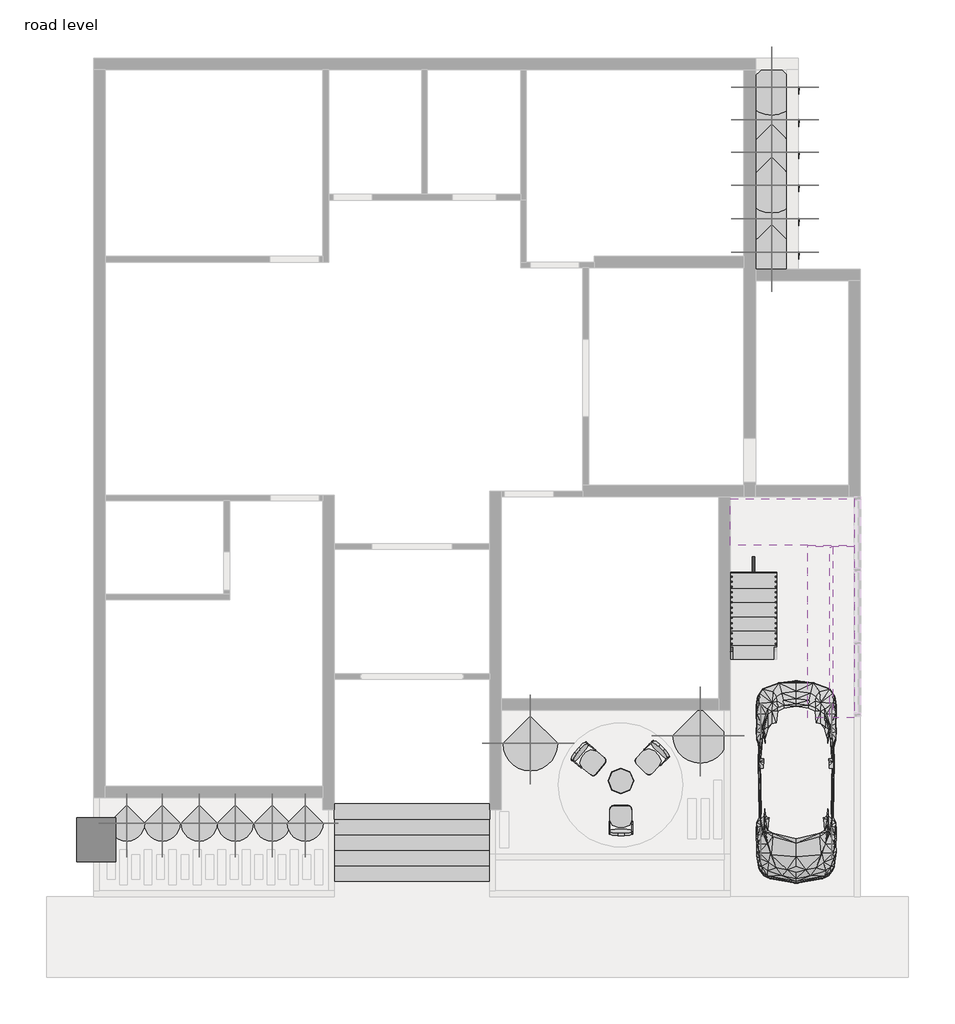
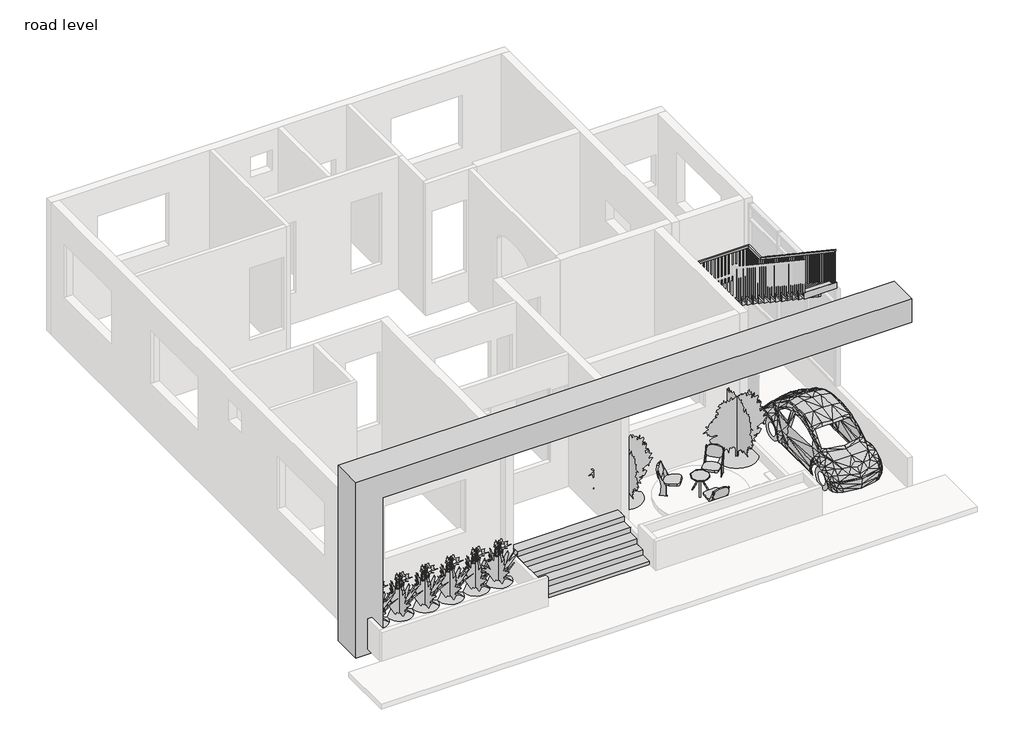
# One storey, part 3 of 3: 14 geographic elements, 6 furniture elements, 2 members, 2 stair flights, 1 proxy, 1 railing, 1 slab.
"""IFC4 building model written with IfcOpenShell, lengths in millimetres."""

from ifc_helpers import new_model, si_unit, frame, origin, place, context, project, spatial, polyline, outline, extrude, faceted_brep, transform, mapped, element, save
from components import rpc_beetle_rpc_beetle_31f8b51e, casework_1_casework_1_0b0e07b3, casework_2_casework_2_4a4ec244, furniture_eb3a3c23, furniture_9d41381f, rpc_plant_tropical_5a024449, rpc_plant_tropical_japanese_fern_2_5_15da35ff, rpc_plant_tropical_jungle_flame_3_a18473df, non_monolithic_landing_47fb7adf, stair_flight_c2955f1a, stair_flight_52fba82a

model = new_model("IFC4")

# Units and contexts
model_context = context("Model", 3, world=origin())
ifc_project = project(units=[si_unit("LENGTHUNIT", "METRE", prefix="MILLI")], contexts=[model_context])

# Site, building, storey
site = spatial("IfcSite", under=ifc_project)
building = spatial("IfcBuilding", under=site)
storey = spatial("IfcBuildingStorey", under=building, Name="road level", Elevation=0.0)

# Proxy
placement = place(None, origin())
rpc_beetle_rpc_beetle_shape = rpc_beetle_rpc_beetle_31f8b51e(model_context)
element("IfcBuildingElementProxy", 1, Name="RPC Beetle : RPC Beetle", ObjectType="RPC Beetle : RPC Beetle", at=placement, inside=storey, context=model_context, shape_type="MappedRepresentation", body=[
    mapped(rpc_beetle_rpc_beetle_shape, transform((-6377.2994093, 2324.2737487, 0.0), x_axis=(-1.0, 0.0, 0.0), y_axis=(0.0, -1.0, 0.0), z_axis=(0.0, 0.0, 1.0))),
])

# Furniture
casework_1_casework_1_shape = casework_1_casework_1_0b0e07b3(model_context)
element("IfcFurniture", 2, ObjectType="Casework 1 : Casework 1", at=placement, inside=storey, context=model_context, shape_type="MappedRepresentation", body=[
    mapped(casework_1_casework_1_shape, transform((0.0, 120.65, -1549.4), x_axis=(1.0, 0.0, 0.0), y_axis=(0.0, 1.0, 0.0), z_axis=(0.0, 0.0, 1.0))),
])
casework_2_casework_2_shape = casework_2_casework_2_4a4ec244(model_context)
element("IfcFurniture", 3, ObjectType="Casework 2 : Casework 2", at=placement, inside=storey, context=model_context, shape_type="MappedRepresentation", body=[
    mapped(casework_2_casework_2_shape, transform((0.0, 0.0, 0.0), x_axis=(1.0, 0.0, 0.0), y_axis=(0.0, 1.0, 0.0), z_axis=(0.0, 0.0, 1.0))),
])
furniture_shape = furniture_eb3a3c23(model_context)
element("IfcFurniture", 4, ObjectType="Seating-Auditorium : 18\" x 24\" x 30\"", at=placement, inside=storey, context=model_context, shape_type="MappedRepresentation", body=[
    mapped(furniture_shape, transform((-10501.2884503, 1788.2599183, 127.0), x_axis=(-0.6326906073859195, -0.7744046715546312, 0.0), y_axis=(0.7744046715546312, -0.6326906073859195, 0.0), z_axis=(0.0, 0.0, 1.0))),
])
element("IfcFurniture", 5, ObjectType="Seating-Auditorium : 18\" x 24\" x 30\"", at=placement, inside=storey, context=model_context, shape_type="MappedRepresentation", body=[
    mapped(furniture_shape, transform((-9979.7272781, 134.5837076, 127.0), x_axis=(1.0, 0.0, 0.0), y_axis=(0.0, 1.0, 0.0), z_axis=(0.0, 0.0, 1.0))),
])
element("IfcFurniture", 6, ObjectType="Seating-Auditorium : 18\" x 24\" x 30\"", at=placement, inside=storey, context=model_context, shape_type="MappedRepresentation", body=[
    mapped(furniture_shape, transform((-8958.0647625, 1589.6695414, 127.0), x_axis=(-0.7071067811865437, 0.7071067811865515, 0.0), y_axis=(-0.7071067811865515, -0.7071067811865437, 0.0), z_axis=(0.0, 0.0, 1.0))),
])
furniture_2_shape = furniture_9d41381f(model_context)
element("IfcFurniture", 7, ObjectType="Table-Trio End : 20\" Diameter", at=placement, inside=storey, context=model_context, shape_type="MappedRepresentation", body=[
    mapped(furniture_2_shape, transform((-9818.9994093, 1111.8591175, 127.0), x_axis=(1.0, 0.0, 0.0), y_axis=(0.0, 1.0, 0.0), z_axis=(0.0, 0.0, 1.0))),
])

# Geographic elements
rpc_plant_tropical_shape = rpc_plant_tropical_5a024449(model_context)
element("IfcGeographicElement", 8, ObjectType="RPC Plant - Tropical", at=placement, inside=storey, context=model_context, shape_type="MappedRepresentation", body=[
    mapped(rpc_plant_tropical_shape, transform((-19521.7994093, 285.9237487, 152.4), x_axis=(1.0, 0.0, 0.0), y_axis=(0.0, 1.0, 0.0), z_axis=(0.0, 0.0, 1.0))),
])
element("IfcGeographicElement", 9, ObjectType="RPC Plant - Tropical", at=placement, inside=storey, context=model_context, shape_type="MappedRepresentation", body=[
    mapped(rpc_plant_tropical_shape, transform((-18823.2994093, 285.9237487, 152.4), x_axis=(1.0, 0.0, 0.0), y_axis=(0.0, 1.0, 0.0), z_axis=(0.0, 0.0, 1.0))),
])
element("IfcGeographicElement", 10, ObjectType="RPC Plant - Tropical", at=placement, inside=storey, context=model_context, shape_type="MappedRepresentation", body=[
    mapped(rpc_plant_tropical_shape, transform((-16016.5994093, 285.9237487, 152.4), x_axis=(1.0, 0.0, 0.0), y_axis=(0.0, 1.0, 0.0), z_axis=(0.0, 0.0, 1.0))),
])
element("IfcGeographicElement", 11, ObjectType="RPC Plant - Tropical", at=placement, inside=storey, context=model_context, shape_type="MappedRepresentation", body=[
    mapped(rpc_plant_tropical_shape, transform((-16664.2994093, 285.9237487, 152.4), x_axis=(1.0, 0.0, 0.0), y_axis=(0.0, 1.0, 0.0), z_axis=(0.0, 0.0, 1.0))),
])
element("IfcGeographicElement", 12, ObjectType="RPC Plant - Tropical", at=placement, inside=storey, context=model_context, shape_type="MappedRepresentation", body=[
    mapped(rpc_plant_tropical_shape, transform((-17387.2102356, 285.9237487, 152.4), x_axis=(1.0, 0.0, 0.0), y_axis=(0.0, 1.0, 0.0), z_axis=(0.0, 0.0, 1.0))),
])
element("IfcGeographicElement", 13, ObjectType="RPC Plant - Tropical", at=placement, inside=storey, context=model_context, shape_type="MappedRepresentation", body=[
    mapped(rpc_plant_tropical_shape, transform((-18100.388583, 285.9237487, 152.4), x_axis=(1.0, 0.0, 0.0), y_axis=(0.0, 1.0, 0.0), z_axis=(0.0, 0.0, 1.0))),
])
rpc_plant_tropical_japanese_fern_2_5_shape = rpc_plant_tropical_japanese_fern_2_5_15da35ff(model_context)
element("IfcGeographicElement", 14, ObjectType="RPC Plant - Tropical : Japanese Fern - 2.5'", at=placement, inside=storey, context=model_context, shape_type="MappedRepresentation", body=[
    mapped(rpc_plant_tropical_japanese_fern_2_5_shape, transform((-6859.8994093, 14725.8237487, 127.0), x_axis=(1.0, 0.0, 0.0), y_axis=(0.0, 1.0, 0.0), z_axis=(0.0, 0.0, 1.0))),
])
element("IfcGeographicElement", 15, ObjectType="RPC Plant - Tropical : Japanese Fern - 2.5'", at=placement, inside=storey, context=model_context, shape_type="MappedRepresentation", body=[
    mapped(rpc_plant_tropical_japanese_fern_2_5_shape, transform((-6859.8994093, 14090.8237487, 127.0), x_axis=(1.0, 0.0, 0.0), y_axis=(0.0, 1.0, 0.0), z_axis=(0.0, 0.0, 1.0))),
])
element("IfcGeographicElement", 16, ObjectType="RPC Plant - Tropical : Japanese Fern - 2.5'", at=placement, inside=storey, context=model_context, shape_type="MappedRepresentation", body=[
    mapped(rpc_plant_tropical_japanese_fern_2_5_shape, transform((-6859.8994093, 13455.8237487, 127.0), x_axis=(1.0, 0.0, 0.0), y_axis=(0.0, 1.0, 0.0), z_axis=(0.0, 0.0, 1.0))),
])
element("IfcGeographicElement", 17, ObjectType="RPC Plant - Tropical : Japanese Fern - 2.5'", at=placement, inside=storey, context=model_context, shape_type="MappedRepresentation", body=[
    mapped(rpc_plant_tropical_japanese_fern_2_5_shape, transform((-6859.8994093, 12808.1237487, 127.0), x_axis=(1.0, 0.0, 0.0), y_axis=(0.0, 1.0, 0.0), z_axis=(0.0, 0.0, 1.0))),
])
element("IfcGeographicElement", 18, ObjectType="RPC Plant - Tropical : Japanese Fern - 2.5'", at=placement, inside=storey, context=model_context, shape_type="MappedRepresentation", body=[
    mapped(rpc_plant_tropical_japanese_fern_2_5_shape, transform((-6859.8994093, 12147.7237487, 127.0), x_axis=(1.0, 0.0, 0.0), y_axis=(0.0, 1.0, 0.0), z_axis=(0.0, 0.0, 1.0))),
])
element("IfcGeographicElement", 19, ObjectType="RPC Plant - Tropical : Japanese Fern - 2.5'", at=placement, inside=storey, context=model_context, shape_type="MappedRepresentation", body=[
    mapped(rpc_plant_tropical_japanese_fern_2_5_shape, transform((-6859.8994093, 11487.3237487, 127.0), x_axis=(1.0, 0.0, 0.0), y_axis=(0.0, 1.0, 0.0), z_axis=(0.0, 0.0, 1.0))),
])
rpc_plant_tropical_jungle_flame_3_shape = rpc_plant_tropical_jungle_flame_3_a18473df(model_context)
element("IfcGeographicElement", 20, ObjectType="RPC Plant - Tropical : Jungle Flame - 3'", at=placement, inside=storey, context=model_context, shape_type="MappedRepresentation", body=[
    mapped(rpc_plant_tropical_jungle_flame_3_shape, transform((-11596.9994093, 1848.0237487, 127.0), x_axis=(1.0, 0.0, 0.0), y_axis=(0.0, 1.0, 0.0), z_axis=(0.0, 0.0, 1.0))),
])
element("IfcGeographicElement", 21, ObjectType="RPC Plant - Tropical : Jungle Flame - 3'", at=placement, inside=storey, context=model_context, shape_type="MappedRepresentation", body=[
    mapped(rpc_plant_tropical_jungle_flame_3_shape, transform((-8261.3350514, 2000.4237487, 127.0), x_axis=(1.0, 0.0, 0.0), y_axis=(0.0, 1.0, 0.0), z_axis=(0.0, 0.0, 1.0))),
])

# Members
element("IfcMember", 22, ObjectType="Carriage - 2\" Width", at=placement, inside=storey, context=model_context, shape_type="SweptSolid", body=[
    extrude(outline(polyline([(5734.2237487, 1445.4909091), (5734.2237487, 1347.8221019), (3720.8104853, 0.0), (3530.7737487, 0.0), (3530.7737487, 136.2363636), (3810.1737487, 136.2363636), (3810.1737487, 323.2727273), (4089.5737487, 323.2727273), (4089.5737487, 510.3090909), (4368.9737487, 510.3090909), (4368.9737487, 697.3454545), (4648.3737487, 697.3454545), (4648.3737487, 884.3818182), (4927.7737487, 884.3818182), (4927.7737487, 1071.4181818), (5207.1737487, 1071.4181818), (5207.1737487, 1258.4545455), (5486.5737487, 1258.4545455), (5486.5737487, 1445.4909091), (5734.2237487, 1445.4909091)])), frame((-7240.8994093, 0.0, 0.0), z_axis=(1.0, 0.0, 0.0), x_axis=(0.0, 1.0, 0.0)), (0.0, 0.0, 1.0), 50.8),
])
element("IfcMember", 23, ObjectType="Carriage - 2\" Width", at=placement, inside=storey, context=model_context, shape_type="SweptSolid", body=[
    extrude(outline(polyline([(2381.4237487, 3779.2948292), (2381.4237487, 3876.9636364), (2629.0737487, 3876.9636364), (2629.0737487, 3689.9272727), (2908.4737487, 3689.9272727), (2908.4737487, 3502.8909091), (3187.8737487, 3502.8909091), (3187.8737487, 3315.8545455), (3467.2737487, 3315.8545455), (3467.2737487, 3128.8181818), (3746.6737487, 3128.8181818), (3746.6737487, 2941.7818182), (4026.0737487, 2941.7818182), (4026.0737487, 2754.7454545), (4305.4737487, 2754.7454545), (4305.4737487, 2567.7090909), (4584.8737487, 2567.7090909), (4584.8737487, 2380.6727273), (4864.2737487, 2380.6727273), (4864.2737487, 2193.6363636), (5143.6737487, 2193.6363636), (5143.6737487, 2006.6), (5423.0737487, 2006.6), (5423.0737487, 1819.5636364), (5702.4737487, 1819.5636364), (5702.4737487, 1556.1125978), (2381.4237487, 3779.2948292)])), frame((-5716.8994093, 0.0, 0.0), z_axis=(1.0, 0.0, 0.0), x_axis=(0.0, 1.0, 0.0)), (0.0, 0.0, 1.0), 50.8),
])

# Railing
element("IfcRailing", 24, ObjectType="Handrail - Rectangular", at=placement, inside=storey, context=model_context, shape_type="SolidModel", body=[
    faceted_brep([(-7672.6994093, 3499.0237487, 1101.4363636), (-7672.6994093, 3499.0237487, 1040.3046237), (-7621.8994093, 3499.0237487, 1040.3046237), (-7621.8994093, 3499.0237487, 1101.4363636), (-7672.6994093, 5734.2237487, 2597.7272727), (-7672.6994093, 5749.6575825, 2546.9272727), (-7621.8994093, 5749.6575825, 2546.9272727), (-7621.8994093, 5734.2237487, 2597.7272727), (-7672.6994093, 6648.6237487, 2597.7272727), (-7672.6994093, 6648.6237487, 2546.9272727), (-7621.8994093, 6597.8237487, 2546.9272727), (-7621.8994093, 6597.8237487, 2597.7272727), (-5234.2994093, 6648.6237487, 2597.7272727), (-5234.2994093, 6648.6237487, 2546.9272727), (-5285.0994093, 6597.8237487, 2546.9272727), (-5285.0994093, 6597.8237487, 2597.7272727), (-5234.2994093, 6013.6237487, 2597.7272727), (-5234.2994093, 5998.1899149, 2546.9272727), (-5285.0994093, 5998.1899149, 2546.9272727), (-5285.0994093, 6013.6237487, 2597.7272727), (-5234.2994093, 5734.2237487, 2784.7636364), (-5234.2994093, 5705.9645192, 2742.5492318), (-5285.0994093, 5705.9645192, 2742.5492318), (-5285.0994093, 5734.2237487, 2784.7636364), (-5234.2994093, 2381.4237487, 5029.2), (-5285.0994093, 2381.4237487, 5029.2), (-5285.0994093, 2381.4237487, 4968.06826), (-5234.2994093, 2381.4237487, 4968.06826)], [[[0, 1, 2, 3]], [[1, 0, 4, 5]], [[2, 1, 5, 6]], [[3, 2, 6, 7]], [[0, 3, 7, 4]], [[5, 4, 8, 9]], [[6, 5, 9, 10]], [[7, 6, 10, 11]], [[4, 7, 11, 8]], [[9, 8, 12, 13]], [[10, 9, 13, 14]], [[11, 10, 14, 15]], [[8, 11, 15, 12]], [[13, 12, 16, 17]], [[14, 13, 17, 18]], [[15, 14, 18, 19]], [[12, 15, 19, 16]], [[17, 16, 20, 21]], [[18, 17, 21, 22]], [[19, 18, 22, 23]], [[16, 19, 23, 20]], [[24, 25, 26, 27]], [[21, 20, 24, 27]], [[22, 21, 27, 26]], [[23, 22, 26, 25]], [[20, 23, 25, 24]]]),
    extrude(outline(polyline([(2492.5487487, 4893.6787972), (2492.5487487, 3927.7636364), (2473.4987487, 3927.7636364), (2473.4987487, 4906.4312766), (2492.5487487, 4893.6787972)])), frame((-5269.2244093, 0.0, 0.0), z_axis=(1.0, 0.0, 0.0), x_axis=(0.0, 1.0, 0.0)), (0.0, 0.0, 1.0), 19.05),
    extrude(outline(polyline([(2594.1487487, 4825.6655741), (2594.1487487, 3927.7636364), (2575.0987487, 3927.7636364), (2575.0987487, 4838.4180534), (2594.1487487, 4825.6655741)])), frame((-5269.2244093, 0.0, 0.0), z_axis=(1.0, 0.0, 0.0), x_axis=(0.0, 1.0, 0.0)), (0.0, 0.0, 1.0), 19.05),
    extrude(outline(polyline([(2695.7487487, 4757.6523509), (2695.7487487, 3740.7272727), (2676.6987487, 3740.7272727), (2676.6987487, 4770.4048303), (2695.7487487, 4757.6523509)])), frame((-5269.2244093, 0.0, 0.0), z_axis=(1.0, 0.0, 0.0), x_axis=(0.0, 1.0, 0.0)), (0.0, 0.0, 1.0), 19.05),
    extrude(outline(polyline([(2797.3487487, 4689.6391278), (2797.3487487, 3740.7272727), (2778.2987487, 3740.7272727), (2778.2987487, 4702.3916071), (2797.3487487, 4689.6391278)])), frame((-5269.2244093, 0.0, 0.0), z_axis=(1.0, 0.0, 0.0), x_axis=(0.0, 1.0, 0.0)), (0.0, 0.0, 1.0), 19.05),
    extrude(outline(polyline([(2898.9487487, 4621.6259047), (2898.9487487, 3740.7272727), (2879.8987487, 3740.7272727), (2879.8987487, 4634.378384), (2898.9487487, 4621.6259047)])), frame((-5269.2244093, 0.0, 0.0), z_axis=(1.0, 0.0, 0.0), x_axis=(0.0, 1.0, 0.0)), (0.0, 0.0, 1.0), 19.05),
    extrude(outline(polyline([(3000.5487487, 4553.6126815), (3000.5487487, 3553.6909091), (2981.4987487, 3553.6909091), (2981.4987487, 4566.3651609), (3000.5487487, 4553.6126815)])), frame((-5269.2244093, 0.0, 0.0), z_axis=(1.0, 0.0, 0.0), x_axis=(0.0, 1.0, 0.0)), (0.0, 0.0, 1.0), 19.05),
    extrude(outline(polyline([(3102.1487487, 4485.5994584), (3102.1487487, 3553.6909091), (3083.0987487, 3553.6909091), (3083.0987487, 4498.3519377), (3102.1487487, 4485.5994584)])), frame((-5269.2244093, 0.0, 0.0), z_axis=(1.0, 0.0, 0.0), x_axis=(0.0, 1.0, 0.0)), (0.0, 0.0, 1.0), 19.05),
    extrude(outline(polyline([(3203.7487487, 4417.5862352), (3203.7487487, 3553.6909091), (3184.6987487, 3553.6909091), (3184.6987487, 4430.3387146), (3203.7487487, 4417.5862352)])), frame((-5269.2244093, 0.0, 0.0), z_axis=(1.0, 0.0, 0.0), x_axis=(0.0, 1.0, 0.0)), (0.0, 0.0, 1.0), 19.05),
    extrude(outline(polyline([(3305.3487487, 4349.5730121), (3305.3487487, 3366.6545455), (3286.2987487, 3366.6545455), (3286.2987487, 4362.3254914), (3305.3487487, 4349.5730121)])), frame((-5269.2244093, 0.0, 0.0), z_axis=(1.0, 0.0, 0.0), x_axis=(0.0, 1.0, 0.0)), (0.0, 0.0, 1.0), 19.05),
    extrude(outline(polyline([(3406.9487487, 4281.559789), (3406.9487487, 3366.6545455), (3387.8987487, 3366.6545455), (3387.8987487, 4294.3122683), (3406.9487487, 4281.559789)])), frame((-5269.2244093, 0.0, 0.0), z_axis=(1.0, 0.0, 0.0), x_axis=(0.0, 1.0, 0.0)), (0.0, 0.0, 1.0), 19.05),
    extrude(outline(polyline([(3508.5487487, 4213.5465658), (3508.5487487, 3366.6545455), (3489.4987487, 3366.6545455), (3489.4987487, 4226.2990452), (3508.5487487, 4213.5465658)])), frame((-5269.2244093, 0.0, 0.0), z_axis=(1.0, 0.0, 0.0), x_axis=(0.0, 1.0, 0.0)), (0.0, 0.0, 1.0), 19.05),
    extrude(outline(polyline([(3610.1487487, 4145.5333427), (3610.1487487, 3179.6181818), (3591.0987487, 3179.6181818), (3591.0987487, 4158.285822), (3610.1487487, 4145.5333427)])), frame((-5269.2244093, 0.0, 0.0), z_axis=(1.0, 0.0, 0.0), x_axis=(0.0, 1.0, 0.0)), (0.0, 0.0, 1.0), 19.05),
    extrude(outline(polyline([(3711.7487487, 4077.5201195), (3711.7487487, 3179.6181818), (3692.6987487, 3179.6181818), (3692.6987487, 4090.2725989), (3711.7487487, 4077.5201195)])), frame((-5269.2244093, 0.0, 0.0), z_axis=(1.0, 0.0, 0.0), x_axis=(0.0, 1.0, 0.0)), (0.0, 0.0, 1.0), 19.05),
    extrude(outline(polyline([(3813.3487487, 4009.5068964), (3813.3487487, 2992.5818182), (3794.2987487, 2992.5818182), (3794.2987487, 4022.2593757), (3813.3487487, 4009.5068964)])), frame((-5269.2244093, 0.0, 0.0), z_axis=(1.0, 0.0, 0.0), x_axis=(0.0, 1.0, 0.0)), (0.0, 0.0, 1.0), 19.05),
    extrude(outline(polyline([(3914.9487487, 3941.4936733), (3914.9487487, 2992.5818182), (3895.8987487, 2992.5818182), (3895.8987487, 3954.2461526), (3914.9487487, 3941.4936733)])), frame((-5269.2244093, 0.0, 0.0), z_axis=(1.0, 0.0, 0.0), x_axis=(0.0, 1.0, 0.0)), (0.0, 0.0, 1.0), 19.05),
    extrude(outline(polyline([(4016.5487487, 3873.4804501), (4016.5487487, 2992.5818182), (3997.4987487, 2992.5818182), (3997.4987487, 3886.2329295), (4016.5487487, 3873.4804501)])), frame((-5269.2244093, 0.0, 0.0), z_axis=(1.0, 0.0, 0.0), x_axis=(0.0, 1.0, 0.0)), (0.0, 0.0, 1.0), 19.05),
    extrude(outline(polyline([(4118.1487487, 3805.467227), (4118.1487487, 2805.5454545), (4099.0987487, 2805.5454545), (4099.0987487, 3818.2197063), (4118.1487487, 3805.467227)])), frame((-5269.2244093, 0.0, 0.0), z_axis=(1.0, 0.0, 0.0), x_axis=(0.0, 1.0, 0.0)), (0.0, 0.0, 1.0), 19.05),
    extrude(outline(polyline([(4219.7487487, 3737.4540038), (4219.7487487, 2805.5454545), (4200.6987487, 2805.5454545), (4200.6987487, 3750.2064832), (4219.7487487, 3737.4540038)])), frame((-5269.2244093, 0.0, 0.0), z_axis=(1.0, 0.0, 0.0), x_axis=(0.0, 1.0, 0.0)), (0.0, 0.0, 1.0), 19.05),
    extrude(outline(polyline([(4321.3487487, 3669.4407807), (4321.3487487, 2805.5454545), (4302.2987487, 2805.5454545), (4302.2987487, 3682.19326), (4321.3487487, 3669.4407807)])), frame((-5269.2244093, 0.0, 0.0), z_axis=(1.0, 0.0, 0.0), x_axis=(0.0, 1.0, 0.0)), (0.0, 0.0, 1.0), 19.05),
    extrude(outline(polyline([(4422.9487487, 3601.4275576), (4422.9487487, 2618.5090909), (4403.8987487, 2618.5090909), (4403.8987487, 3614.1800369), (4422.9487487, 3601.4275576)])), frame((-5269.2244093, 0.0, 0.0), z_axis=(1.0, 0.0, 0.0), x_axis=(0.0, 1.0, 0.0)), (0.0, 0.0, 1.0), 19.05),
    extrude(outline(polyline([(4524.5487487, 3533.4143344), (4524.5487487, 2618.5090909), (4505.4987487, 2618.5090909), (4505.4987487, 3546.1668138), (4524.5487487, 3533.4143344)])), frame((-5269.2244093, 0.0, 0.0), z_axis=(1.0, 0.0, 0.0), x_axis=(0.0, 1.0, 0.0)), (0.0, 0.0, 1.0), 19.05),
    extrude(outline(polyline([(4626.1487487, 3465.4011113), (4626.1487487, 2618.5090909), (4607.0987487, 2618.5090909), (4607.0987487, 3478.1535906), (4626.1487487, 3465.4011113)])), frame((-5269.2244093, 0.0, 0.0), z_axis=(1.0, 0.0, 0.0), x_axis=(0.0, 1.0, 0.0)), (0.0, 0.0, 1.0), 19.05),
    extrude(outline(polyline([(4727.7487487, 3397.3878881), (4727.7487487, 2431.4727273), (4708.6987487, 2431.4727273), (4708.6987487, 3410.1403675), (4727.7487487, 3397.3878881)])), frame((-5269.2244093, 0.0, 0.0), z_axis=(1.0, 0.0, 0.0), x_axis=(0.0, 1.0, 0.0)), (0.0, 0.0, 1.0), 19.05),
    extrude(outline(polyline([(4829.3487487, 3329.374665), (4829.3487487, 2431.4727273), (4810.2987487, 2431.4727273), (4810.2987487, 3342.1271443), (4829.3487487, 3329.374665)])), frame((-5269.2244093, 0.0, 0.0), z_axis=(1.0, 0.0, 0.0), x_axis=(0.0, 1.0, 0.0)), (0.0, 0.0, 1.0), 19.05),
    extrude(outline(polyline([(4930.9487487, 3261.3614419), (4930.9487487, 2244.4363636), (4911.8987487, 2244.4363636), (4911.8987487, 3274.1139212), (4930.9487487, 3261.3614419)])), frame((-5269.2244093, 0.0, 0.0), z_axis=(1.0, 0.0, 0.0), x_axis=(0.0, 1.0, 0.0)), (0.0, 0.0, 1.0), 19.05),
    extrude(outline(polyline([(5032.5487487, 3193.3482187), (5032.5487487, 2244.4363636), (5013.4987487, 2244.4363636), (5013.4987487, 3206.1006981), (5032.5487487, 3193.3482187)])), frame((-5269.2244093, 0.0, 0.0), z_axis=(1.0, 0.0, 0.0), x_axis=(0.0, 1.0, 0.0)), (0.0, 0.0, 1.0), 19.05),
    extrude(outline(polyline([(5134.1487487, 3125.3349956), (5134.1487487, 2244.4363636), (5115.0987487, 2244.4363636), (5115.0987487, 3138.0874749), (5134.1487487, 3125.3349956)])), frame((-5269.2244093, 0.0, 0.0), z_axis=(1.0, 0.0, 0.0), x_axis=(0.0, 1.0, 0.0)), (0.0, 0.0, 1.0), 19.05),
    extrude(outline(polyline([(5235.7487487, 3057.3217724), (5235.7487487, 2057.4), (5216.6987487, 2057.4), (5216.6987487, 3070.0742518), (5235.7487487, 3057.3217724)])), frame((-5269.2244093, 0.0, 0.0), z_axis=(1.0, 0.0, 0.0), x_axis=(0.0, 1.0, 0.0)), (0.0, 0.0, 1.0), 19.05),
    extrude(outline(polyline([(5337.3487487, 2989.3085493), (5337.3487487, 2057.4), (5318.2987487, 2057.4), (5318.2987487, 3002.0610286), (5337.3487487, 2989.3085493)])), frame((-5269.2244093, 0.0, 0.0), z_axis=(1.0, 0.0, 0.0), x_axis=(0.0, 1.0, 0.0)), (0.0, 0.0, 1.0), 19.05),
    extrude(outline(polyline([(5438.9487487, 2921.2953262), (5438.9487487, 2057.4), (5419.8987487, 2057.4), (5419.8987487, 2934.0478055), (5438.9487487, 2921.2953262)])), frame((-5269.2244093, 0.0, 0.0), z_axis=(1.0, 0.0, 0.0), x_axis=(0.0, 1.0, 0.0)), (0.0, 0.0, 1.0), 19.05),
    extrude(outline(polyline([(5540.5487487, 2853.282103), (5540.5487487, 1870.3636364), (5521.4987487, 1870.3636364), (5521.4987487, 2866.0345824), (5540.5487487, 2853.282103)])), frame((-5269.2244093, 0.0, 0.0), z_axis=(1.0, 0.0, 0.0), x_axis=(0.0, 1.0, 0.0)), (0.0, 0.0, 1.0), 19.05),
    extrude(outline(polyline([(5642.1487487, 2785.2688799), (5642.1487487, 1870.3636364), (5623.0987487, 1870.3636364), (5623.0987487, 2798.0213592), (5642.1487487, 2785.2688799)])), frame((-5269.2244093, 0.0, 0.0), z_axis=(1.0, 0.0, 0.0), x_axis=(0.0, 1.0, 0.0)), (0.0, 0.0, 1.0), 19.05),
    extrude(outline(polyline([(5819.9487487, 2666.2457394), (5819.9487487, 1683.3272727), (5800.8987487, 1683.3272727), (5800.8987487, 2678.9982187), (5819.9487487, 2666.2457394)])), frame((-5269.2244093, 0.0, 0.0), z_axis=(1.0, 0.0, 0.0), x_axis=(0.0, 1.0, 0.0)), (0.0, 0.0, 1.0), 19.05),
    extrude(outline(polyline([(5921.5487487, 2598.2325162), (5921.5487487, 1683.3272727), (5902.4987487, 1683.3272727), (5902.4987487, 2610.9849956), (5921.5487487, 2598.2325162)])), frame((-5269.2244093, 0.0, 0.0), z_axis=(1.0, 0.0, 0.0), x_axis=(0.0, 1.0, 0.0)), (0.0, 0.0, 1.0), 19.05),
    extrude(outline(polyline([(-5250.1744093, 6023.1487487), (-5250.1744093, 6004.0987487), (-5269.2244093, 6004.0987487), (-5269.2244093, 6023.1487487), (-5250.1744093, 6023.1487487)])), frame((0.0, 0.0, 1683.3272727), z_axis=(0.0, 0.0, 1.0), x_axis=(1.0, 0.0, 0.0)), (0.0, 0.0, 1.0), 863.6),
    extrude(outline(polyline([(-5250.1744093, 6124.7487487), (-5250.1744093, 6105.6987487), (-5269.2244093, 6105.6987487), (-5269.2244093, 6124.7487487), (-5250.1744093, 6124.7487487)])), frame((0.0, 0.0, 1683.3272727), z_axis=(0.0, 0.0, 1.0), x_axis=(1.0, 0.0, 0.0)), (0.0, 0.0, 1.0), 863.6),
    extrude(outline(polyline([(-5250.1744093, 6226.3487487), (-5250.1744093, 6207.2987487), (-5269.2244093, 6207.2987487), (-5269.2244093, 6226.3487487), (-5250.1744093, 6226.3487487)])), frame((0.0, 0.0, 1683.3272727), z_axis=(0.0, 0.0, 1.0), x_axis=(1.0, 0.0, 0.0)), (0.0, 0.0, 1.0), 863.6),
    extrude(outline(polyline([(-5250.1744093, 6327.9487487), (-5250.1744093, 6308.8987487), (-5269.2244093, 6308.8987487), (-5269.2244093, 6327.9487487), (-5250.1744093, 6327.9487487)])), frame((0.0, 0.0, 1683.3272727), z_axis=(0.0, 0.0, 1.0), x_axis=(1.0, 0.0, 0.0)), (0.0, 0.0, 1.0), 863.6),
    extrude(outline(polyline([(-5250.1744093, 6429.5487487), (-5250.1744093, 6410.4987487), (-5269.2244093, 6410.4987487), (-5269.2244093, 6429.5487487), (-5250.1744093, 6429.5487487)])), frame((0.0, 0.0, 1683.3272727), z_axis=(0.0, 0.0, 1.0), x_axis=(1.0, 0.0, 0.0)), (0.0, 0.0, 1.0), 863.6),
    extrude(outline(polyline([(-5250.1744093, 6531.1487487), (-5250.1744093, 6512.0987487), (-5269.2244093, 6512.0987487), (-5269.2244093, 6531.1487487), (-5250.1744093, 6531.1487487)])), frame((0.0, 0.0, 1683.3272727), z_axis=(0.0, 0.0, 1.0), x_axis=(1.0, 0.0, 0.0)), (0.0, 0.0, 1.0), 863.6),
    extrude(outline(polyline([(-5320.0244093, 6632.7487487), (-5300.9744093, 6632.7487487), (-5300.9744093, 6613.6987487), (-5320.0244093, 6613.6987487), (-5320.0244093, 6632.7487487)])), frame((0.0, 0.0, 1683.3272727), z_axis=(0.0, 0.0, 1.0), x_axis=(1.0, 0.0, 0.0)), (0.0, 0.0, 1.0), 863.6),
    extrude(outline(polyline([(-5421.6244093, 6632.7487487), (-5402.5744093, 6632.7487487), (-5402.5744093, 6613.6987487), (-5421.6244093, 6613.6987487), (-5421.6244093, 6632.7487487)])), frame((0.0, 0.0, 1683.3272727), z_axis=(0.0, 0.0, 1.0), x_axis=(1.0, 0.0, 0.0)), (0.0, 0.0, 1.0), 863.6),
    extrude(outline(polyline([(-5523.2244093, 6632.7487487), (-5504.1744093, 6632.7487487), (-5504.1744093, 6613.6987487), (-5523.2244093, 6613.6987487), (-5523.2244093, 6632.7487487)])), frame((0.0, 0.0, 1683.3272727), z_axis=(0.0, 0.0, 1.0), x_axis=(1.0, 0.0, 0.0)), (0.0, 0.0, 1.0), 863.6),
    extrude(outline(polyline([(-5624.8244093, 6632.7487487), (-5605.7744093, 6632.7487487), (-5605.7744093, 6613.6987487), (-5624.8244093, 6613.6987487), (-5624.8244093, 6632.7487487)])), frame((0.0, 0.0, 1683.3272727), z_axis=(0.0, 0.0, 1.0), x_axis=(1.0, 0.0, 0.0)), (0.0, 0.0, 1.0), 863.6),
    extrude(outline(polyline([(-5726.4244093, 6632.7487487), (-5707.3744093, 6632.7487487), (-5707.3744093, 6613.6987487), (-5726.4244093, 6613.6987487), (-5726.4244093, 6632.7487487)])), frame((0.0, 0.0, 1683.3272727), z_axis=(0.0, 0.0, 1.0), x_axis=(1.0, 0.0, 0.0)), (0.0, 0.0, 1.0), 863.6),
    extrude(outline(polyline([(-5828.0244093, 6632.7487487), (-5808.9744093, 6632.7487487), (-5808.9744093, 6613.6987487), (-5828.0244093, 6613.6987487), (-5828.0244093, 6632.7487487)])), frame((0.0, 0.0, 1683.3272727), z_axis=(0.0, 0.0, 1.0), x_axis=(1.0, 0.0, 0.0)), (0.0, 0.0, 1.0), 863.6),
    extrude(outline(polyline([(-5929.6244093, 6632.7487487), (-5910.5744093, 6632.7487487), (-5910.5744093, 6613.6987487), (-5929.6244093, 6613.6987487), (-5929.6244093, 6632.7487487)])), frame((0.0, 0.0, 1683.3272727), z_axis=(0.0, 0.0, 1.0), x_axis=(1.0, 0.0, 0.0)), (0.0, 0.0, 1.0), 863.6),
    extrude(outline(polyline([(-6031.2244093, 6632.7487487), (-6012.1744093, 6632.7487487), (-6012.1744093, 6613.6987487), (-6031.2244093, 6613.6987487), (-6031.2244093, 6632.7487487)])), frame((0.0, 0.0, 1683.3272727), z_axis=(0.0, 0.0, 1.0), x_axis=(1.0, 0.0, 0.0)), (0.0, 0.0, 1.0), 863.6),
    extrude(outline(polyline([(-6132.8244093, 6632.7487487), (-6113.7744093, 6632.7487487), (-6113.7744093, 6613.6987487), (-6132.8244093, 6613.6987487), (-6132.8244093, 6632.7487487)])), frame((0.0, 0.0, 1683.3272727), z_axis=(0.0, 0.0, 1.0), x_axis=(1.0, 0.0, 0.0)), (0.0, 0.0, 1.0), 863.6),
    extrude(outline(polyline([(-6234.4244093, 6632.7487487), (-6215.3744093, 6632.7487487), (-6215.3744093, 6613.6987487), (-6234.4244093, 6613.6987487), (-6234.4244093, 6632.7487487)])), frame((0.0, 0.0, 1683.3272727), z_axis=(0.0, 0.0, 1.0), x_axis=(1.0, 0.0, 0.0)), (0.0, 0.0, 1.0), 863.6),
    extrude(outline(polyline([(-6336.0244093, 6632.7487487), (-6316.9744093, 6632.7487487), (-6316.9744093, 6613.6987487), (-6336.0244093, 6613.6987487), (-6336.0244093, 6632.7487487)])), frame((0.0, 0.0, 1683.3272727), z_axis=(0.0, 0.0, 1.0), x_axis=(1.0, 0.0, 0.0)), (0.0, 0.0, 1.0), 863.6),
    extrude(outline(polyline([(-6437.6244093, 6632.7487487), (-6418.5744093, 6632.7487487), (-6418.5744093, 6613.6987487), (-6437.6244093, 6613.6987487), (-6437.6244093, 6632.7487487)])), frame((0.0, 0.0, 1683.3272727), z_axis=(0.0, 0.0, 1.0), x_axis=(1.0, 0.0, 0.0)), (0.0, 0.0, 1.0), 863.6),
    extrude(outline(polyline([(-6539.2244093, 6632.7487487), (-6520.1744093, 6632.7487487), (-6520.1744093, 6613.6987487), (-6539.2244093, 6613.6987487), (-6539.2244093, 6632.7487487)])), frame((0.0, 0.0, 1683.3272727), z_axis=(0.0, 0.0, 1.0), x_axis=(1.0, 0.0, 0.0)), (0.0, 0.0, 1.0), 863.6),
    extrude(outline(polyline([(-6640.8244093, 6632.7487487), (-6621.7744093, 6632.7487487), (-6621.7744093, 6613.6987487), (-6640.8244093, 6613.6987487), (-6640.8244093, 6632.7487487)])), frame((0.0, 0.0, 1683.3272727), z_axis=(0.0, 0.0, 1.0), x_axis=(1.0, 0.0, 0.0)), (0.0, 0.0, 1.0), 863.6),
    extrude(outline(polyline([(-6742.4244093, 6632.7487487), (-6723.3744093, 6632.7487487), (-6723.3744093, 6613.6987487), (-6742.4244093, 6613.6987487), (-6742.4244093, 6632.7487487)])), frame((0.0, 0.0, 1683.3272727), z_axis=(0.0, 0.0, 1.0), x_axis=(1.0, 0.0, 0.0)), (0.0, 0.0, 1.0), 863.6),
    extrude(outline(polyline([(-6844.0244093, 6632.7487487), (-6824.9744093, 6632.7487487), (-6824.9744093, 6613.6987487), (-6844.0244093, 6613.6987487), (-6844.0244093, 6632.7487487)])), frame((0.0, 0.0, 1683.3272727), z_axis=(0.0, 0.0, 1.0), x_axis=(1.0, 0.0, 0.0)), (0.0, 0.0, 1.0), 863.6),
    extrude(outline(polyline([(-6945.6244093, 6632.7487487), (-6926.5744093, 6632.7487487), (-6926.5744093, 6613.6987487), (-6945.6244093, 6613.6987487), (-6945.6244093, 6632.7487487)])), frame((0.0, 0.0, 1683.3272727), z_axis=(0.0, 0.0, 1.0), x_axis=(1.0, 0.0, 0.0)), (0.0, 0.0, 1.0), 863.6),
    extrude(outline(polyline([(-7047.2244093, 6632.7487487), (-7028.1744093, 6632.7487487), (-7028.1744093, 6613.6987487), (-7047.2244093, 6613.6987487), (-7047.2244093, 6632.7487487)])), frame((0.0, 0.0, 1683.3272727), z_axis=(0.0, 0.0, 1.0), x_axis=(1.0, 0.0, 0.0)), (0.0, 0.0, 1.0), 863.6),
    extrude(outline(polyline([(-7148.8244093, 6632.7487487), (-7129.7744093, 6632.7487487), (-7129.7744093, 6613.6987487), (-7148.8244093, 6613.6987487), (-7148.8244093, 6632.7487487)])), frame((0.0, 0.0, 1683.3272727), z_axis=(0.0, 0.0, 1.0), x_axis=(1.0, 0.0, 0.0)), (0.0, 0.0, 1.0), 863.6),
    extrude(outline(polyline([(-7250.4244093, 6632.7487487), (-7231.3744093, 6632.7487487), (-7231.3744093, 6613.6987487), (-7250.4244093, 6613.6987487), (-7250.4244093, 6632.7487487)])), frame((0.0, 0.0, 1683.3272727), z_axis=(0.0, 0.0, 1.0), x_axis=(1.0, 0.0, 0.0)), (0.0, 0.0, 1.0), 863.6),
    extrude(outline(polyline([(-7352.0244093, 6632.7487487), (-7332.9744093, 6632.7487487), (-7332.9744093, 6613.6987487), (-7352.0244093, 6613.6987487), (-7352.0244093, 6632.7487487)])), frame((0.0, 0.0, 1683.3272727), z_axis=(0.0, 0.0, 1.0), x_axis=(1.0, 0.0, 0.0)), (0.0, 0.0, 1.0), 863.6),
    extrude(outline(polyline([(-7453.6244093, 6632.7487487), (-7434.5744093, 6632.7487487), (-7434.5744093, 6613.6987487), (-7453.6244093, 6613.6987487), (-7453.6244093, 6632.7487487)])), frame((0.0, 0.0, 1683.3272727), z_axis=(0.0, 0.0, 1.0), x_axis=(1.0, 0.0, 0.0)), (0.0, 0.0, 1.0), 863.6),
    extrude(outline(polyline([(-7555.2244093, 6632.7487487), (-7536.1744093, 6632.7487487), (-7536.1744093, 6613.6987487), (-7555.2244093, 6613.6987487), (-7555.2244093, 6632.7487487)])), frame((0.0, 0.0, 1683.3272727), z_axis=(0.0, 0.0, 1.0), x_axis=(1.0, 0.0, 0.0)), (0.0, 0.0, 1.0), 863.6),
    extrude(outline(polyline([(-7656.8244093, 6537.4987487), (-7656.8244093, 6556.5487487), (-7637.7744093, 6556.5487487), (-7637.7744093, 6537.4987487), (-7656.8244093, 6537.4987487)])), frame((0.0, 0.0, 1683.3272727), z_axis=(0.0, 0.0, 1.0), x_axis=(1.0, 0.0, 0.0)), (0.0, 0.0, 1.0), 863.6),
    extrude(outline(polyline([(-7656.8244093, 6435.8987487), (-7656.8244093, 6454.9487487), (-7637.7744093, 6454.9487487), (-7637.7744093, 6435.8987487), (-7656.8244093, 6435.8987487)])), frame((0.0, 0.0, 1683.3272727), z_axis=(0.0, 0.0, 1.0), x_axis=(1.0, 0.0, 0.0)), (0.0, 0.0, 1.0), 863.6),
    extrude(outline(polyline([(-7656.8244093, 6334.2987487), (-7656.8244093, 6353.3487487), (-7637.7744093, 6353.3487487), (-7637.7744093, 6334.2987487), (-7656.8244093, 6334.2987487)])), frame((0.0, 0.0, 1683.3272727), z_axis=(0.0, 0.0, 1.0), x_axis=(1.0, 0.0, 0.0)), (0.0, 0.0, 1.0), 863.6),
    extrude(outline(polyline([(-7656.8244093, 6232.6987487), (-7656.8244093, 6251.7487487), (-7637.7744093, 6251.7487487), (-7637.7744093, 6232.6987487), (-7656.8244093, 6232.6987487)])), frame((0.0, 0.0, 1683.3272727), z_axis=(0.0, 0.0, 1.0), x_axis=(1.0, 0.0, 0.0)), (0.0, 0.0, 1.0), 863.6),
    extrude(outline(polyline([(-7656.8244093, 6131.0987487), (-7656.8244093, 6150.1487487), (-7637.7744093, 6150.1487487), (-7637.7744093, 6131.0987487), (-7656.8244093, 6131.0987487)])), frame((0.0, 0.0, 1683.3272727), z_axis=(0.0, 0.0, 1.0), x_axis=(1.0, 0.0, 0.0)), (0.0, 0.0, 1.0), 863.6),
    extrude(outline(polyline([(-7656.8244093, 6029.4987487), (-7656.8244093, 6048.5487487), (-7637.7744093, 6048.5487487), (-7637.7744093, 6029.4987487), (-7656.8244093, 6029.4987487)])), frame((0.0, 0.0, 1683.3272727), z_axis=(0.0, 0.0, 1.0), x_axis=(1.0, 0.0, 0.0)), (0.0, 0.0, 1.0), 863.6),
    extrude(outline(polyline([(-7656.8244093, 5927.8987487), (-7656.8244093, 5946.9487487), (-7637.7744093, 5946.9487487), (-7637.7744093, 5927.8987487), (-7656.8244093, 5927.8987487)])), frame((0.0, 0.0, 1683.3272727), z_axis=(0.0, 0.0, 1.0), x_axis=(1.0, 0.0, 0.0)), (0.0, 0.0, 1.0), 863.6),
    extrude(outline(polyline([(-7656.8244093, 5826.2987487), (-7656.8244093, 5845.3487487), (-7637.7744093, 5845.3487487), (-7637.7744093, 5826.2987487), (-7656.8244093, 5826.2987487)])), frame((0.0, 0.0, 1683.3272727), z_axis=(0.0, 0.0, 1.0), x_axis=(1.0, 0.0, 0.0)), (0.0, 0.0, 1.0), 863.6),
    extrude(outline(polyline([(5642.1487487, 2474.9585493), (5642.1487487, 1496.2909091), (5623.0987487, 1496.2909091), (5623.0987487, 2462.20607), (5642.1487487, 2474.9585493)])), frame((-7656.8244093, 0.0, 0.0), z_axis=(1.0, 0.0, 0.0), x_axis=(0.0, 1.0, 0.0)), (0.0, 0.0, 1.0), 19.05),
    extrude(outline(polyline([(5540.5487487, 2406.9453262), (5540.5487487, 1496.2909091), (5521.4987487, 1496.2909091), (5521.4987487, 2394.1928468), (5540.5487487, 2406.9453262)])), frame((-7656.8244093, 0.0, 0.0), z_axis=(1.0, 0.0, 0.0), x_axis=(0.0, 1.0, 0.0)), (0.0, 0.0, 1.0), 19.05),
    extrude(outline(polyline([(5438.9487487, 2338.932103), (5438.9487487, 1309.2545455), (5419.8987487, 1309.2545455), (5419.8987487, 2326.1796237), (5438.9487487, 2338.932103)])), frame((-7656.8244093, 0.0, 0.0), z_axis=(1.0, 0.0, 0.0), x_axis=(0.0, 1.0, 0.0)), (0.0, 0.0, 1.0), 19.05),
    extrude(outline(polyline([(5337.3487487, 2270.9188799), (5337.3487487, 1309.2545455), (5318.2987487, 1309.2545455), (5318.2987487, 2258.1664005), (5337.3487487, 2270.9188799)])), frame((-7656.8244093, 0.0, 0.0), z_axis=(1.0, 0.0, 0.0), x_axis=(0.0, 1.0, 0.0)), (0.0, 0.0, 1.0), 19.05),
    extrude(outline(polyline([(5235.7487487, 2202.9056567), (5235.7487487, 1309.2545455), (5216.6987487, 1309.2545455), (5216.6987487, 2190.1531774), (5235.7487487, 2202.9056567)])), frame((-7656.8244093, 0.0, 0.0), z_axis=(1.0, 0.0, 0.0), x_axis=(0.0, 1.0, 0.0)), (0.0, 0.0, 1.0), 19.05),
    extrude(outline(polyline([(5134.1487487, 2134.8924336), (5134.1487487, 1122.2181818), (5115.0987487, 1122.2181818), (5115.0987487, 2122.1399543), (5134.1487487, 2134.8924336)])), frame((-7656.8244093, 0.0, 0.0), z_axis=(1.0, 0.0, 0.0), x_axis=(0.0, 1.0, 0.0)), (0.0, 0.0, 1.0), 19.05),
    extrude(outline(polyline([(5032.5487487, 2066.8792105), (5032.5487487, 1122.2181818), (5013.4987487, 1122.2181818), (5013.4987487, 2054.1267311), (5032.5487487, 2066.8792105)])), frame((-7656.8244093, 0.0, 0.0), z_axis=(1.0, 0.0, 0.0), x_axis=(0.0, 1.0, 0.0)), (0.0, 0.0, 1.0), 19.05),
    extrude(outline(polyline([(4930.9487487, 1998.8659873), (4930.9487487, 1122.2181818), (4911.8987487, 1122.2181818), (4911.8987487, 1986.113508), (4930.9487487, 1998.8659873)])), frame((-7656.8244093, 0.0, 0.0), z_axis=(1.0, 0.0, 0.0), x_axis=(0.0, 1.0, 0.0)), (0.0, 0.0, 1.0), 19.05),
    extrude(outline(polyline([(4829.3487487, 1930.8527642), (4829.3487487, 935.1818182), (4810.2987487, 935.1818182), (4810.2987487, 1918.1002848), (4829.3487487, 1930.8527642)])), frame((-7656.8244093, 0.0, 0.0), z_axis=(1.0, 0.0, 0.0), x_axis=(0.0, 1.0, 0.0)), (0.0, 0.0, 1.0), 19.05),
    extrude(outline(polyline([(4727.7487487, 1862.839541), (4727.7487487, 935.1818182), (4708.6987487, 935.1818182), (4708.6987487, 1850.0870617), (4727.7487487, 1862.839541)])), frame((-7656.8244093, 0.0, 0.0), z_axis=(1.0, 0.0, 0.0), x_axis=(0.0, 1.0, 0.0)), (0.0, 0.0, 1.0), 19.05),
    extrude(outline(polyline([(4626.1487487, 1794.8263179), (4626.1487487, 935.1818182), (4607.0987487, 935.1818182), (4607.0987487, 1782.0738386), (4626.1487487, 1794.8263179)])), frame((-7656.8244093, 0.0, 0.0), z_axis=(1.0, 0.0, 0.0), x_axis=(0.0, 1.0, 0.0)), (0.0, 0.0, 1.0), 19.05),
    extrude(outline(polyline([(4524.5487487, 1726.8130948), (4524.5487487, 748.1454545), (4505.4987487, 748.1454545), (4505.4987487, 1714.0606154), (4524.5487487, 1726.8130948)])), frame((-7656.8244093, 0.0, 0.0), z_axis=(1.0, 0.0, 0.0), x_axis=(0.0, 1.0, 0.0)), (0.0, 0.0, 1.0), 19.05),
    extrude(outline(polyline([(4422.9487487, 1658.7998716), (4422.9487487, 748.1454545), (4403.8987487, 748.1454545), (4403.8987487, 1646.0473923), (4422.9487487, 1658.7998716)])), frame((-7656.8244093, 0.0, 0.0), z_axis=(1.0, 0.0, 0.0), x_axis=(0.0, 1.0, 0.0)), (0.0, 0.0, 1.0), 19.05),
    extrude(outline(polyline([(4321.3487487, 1590.7866485), (4321.3487487, 561.1090909), (4302.2987487, 561.1090909), (4302.2987487, 1578.0341691), (4321.3487487, 1590.7866485)])), frame((-7656.8244093, 0.0, 0.0), z_axis=(1.0, 0.0, 0.0), x_axis=(0.0, 1.0, 0.0)), (0.0, 0.0, 1.0), 19.05),
    extrude(outline(polyline([(4219.7487487, 1522.7734253), (4219.7487487, 561.1090909), (4200.6987487, 561.1090909), (4200.6987487, 1510.020946), (4219.7487487, 1522.7734253)])), frame((-7656.8244093, 0.0, 0.0), z_axis=(1.0, 0.0, 0.0), x_axis=(0.0, 1.0, 0.0)), (0.0, 0.0, 1.0), 19.05),
    extrude(outline(polyline([(4118.1487487, 1454.7602022), (4118.1487487, 561.1090909), (4099.0987487, 561.1090909), (4099.0987487, 1442.0077229), (4118.1487487, 1454.7602022)])), frame((-7656.8244093, 0.0, 0.0), z_axis=(1.0, 0.0, 0.0), x_axis=(0.0, 1.0, 0.0)), (0.0, 0.0, 1.0), 19.05),
    extrude(outline(polyline([(4016.5487487, 1386.746979), (4016.5487487, 374.0727273), (3997.4987487, 374.0727273), (3997.4987487, 1373.9944997), (4016.5487487, 1386.746979)])), frame((-7656.8244093, 0.0, 0.0), z_axis=(1.0, 0.0, 0.0), x_axis=(0.0, 1.0, 0.0)), (0.0, 0.0, 1.0), 19.05),
    extrude(outline(polyline([(3914.9487487, 1318.7337559), (3914.9487487, 374.0727273), (3895.8987487, 374.0727273), (3895.8987487, 1305.9812766), (3914.9487487, 1318.7337559)])), frame((-7656.8244093, 0.0, 0.0), z_axis=(1.0, 0.0, 0.0), x_axis=(0.0, 1.0, 0.0)), (0.0, 0.0, 1.0), 19.05),
    extrude(outline(polyline([(3813.3487487, 1250.7205328), (3813.3487487, 374.0727273), (3794.2987487, 374.0727273), (3794.2987487, 1237.9680534), (3813.3487487, 1250.7205328)])), frame((-7656.8244093, 0.0, 0.0), z_axis=(1.0, 0.0, 0.0), x_axis=(0.0, 1.0, 0.0)), (0.0, 0.0, 1.0), 19.05),
    extrude(outline(polyline([(3711.7487487, 1182.7073096), (3711.7487487, 187.0363636), (3692.6987487, 187.0363636), (3692.6987487, 1169.9548303), (3711.7487487, 1182.7073096)])), frame((-7656.8244093, 0.0, 0.0), z_axis=(1.0, 0.0, 0.0), x_axis=(0.0, 1.0, 0.0)), (0.0, 0.0, 1.0), 19.05),
    extrude(outline(polyline([(3610.1487487, 1114.6940865), (3610.1487487, 187.0363636), (3591.0987487, 187.0363636), (3591.0987487, 1101.9416071), (3610.1487487, 1114.6940865)])), frame((-7656.8244093, 0.0, 0.0), z_axis=(1.0, 0.0, 0.0), x_axis=(0.0, 1.0, 0.0)), (0.0, 0.0, 1.0), 19.05),
    extrude(outline(polyline([(5743.7487487, 2717.2556567), (5743.7487487, 1683.3272727), (5724.6987487, 1683.3272727), (5724.6987487, 2730.0081361), (5743.7487487, 2717.2556567)])), frame((-5269.2244093, 0.0, 0.0), z_axis=(1.0, 0.0, 0.0), x_axis=(0.0, 1.0, 0.0)), (0.0, 0.0, 1.0), 19.05),
    extrude(outline(polyline([(-5269.2244093, 6632.7487487), (-5250.1744093, 6632.7487487), (-5250.1744093, 6613.6987487), (-5269.2244093, 6613.6987487), (-5269.2244093, 6632.7487487)])), frame((0.0, 0.0, 1683.3272727), z_axis=(0.0, 0.0, 1.0), x_axis=(1.0, 0.0, 0.0)), (0.0, 0.0, 1.0), 863.6),
    extrude(outline(polyline([(-7656.8244093, 6613.6987487), (-7656.8244093, 6632.7487487), (-7637.7744093, 6632.7487487), (-7637.7744093, 6613.6987487), (-7656.8244093, 6613.6987487)])), frame((0.0, 0.0, 1683.3272727), z_axis=(0.0, 0.0, 1.0), x_axis=(1.0, 0.0, 0.0)), (0.0, 0.0, 1.0), 863.6),
    extrude(outline(polyline([(5743.7487487, 2542.9717724), (5743.7487487, 1683.3272727), (5724.6987487, 1683.3272727), (5724.6987487, 2530.2192931), (5743.7487487, 2542.9717724)])), frame((-7656.8244093, 0.0, 0.0), z_axis=(1.0, 0.0, 0.0), x_axis=(0.0, 1.0, 0.0)), (0.0, 0.0, 1.0), 19.05),
    extrude(outline(polyline([(2400.4737487, 4955.3157807), (2400.4737487, 3927.7636364), (2381.4237487, 3927.7636364), (2381.4237487, 4968.06826), (2400.4737487, 4955.3157807)])), frame((-5269.2244093, 0.0, 0.0), z_axis=(1.0, 0.0, 0.0), x_axis=(0.0, 1.0, 0.0)), (0.0, 0.0, 1.0), 19.05),
    extrude(outline(polyline([(3518.0737487, 1053.057103), (3518.0737487, 187.0363636), (3499.0237487, 187.0363636), (3499.0237487, 1040.3046237), (3518.0737487, 1053.057103)])), frame((-7656.8244093, 0.0, 0.0), z_axis=(1.0, 0.0, 0.0), x_axis=(0.0, 1.0, 0.0)), (0.0, 0.0, 1.0), 19.05),
])

# Slab
non_monolithic_landing_shape = non_monolithic_landing_47fb7adf(model_context)
element("IfcSlab", 25, ObjectType="Non-Monolithic Landing", at=placement, inside=storey, context=model_context, shape_type="MappedRepresentation", body=[
    mapped(non_monolithic_landing_shape, transform((0.0, 0.0, 0.0), x_axis=(1.0, 0.0, 0.0), y_axis=(0.0, 1.0, 0.0), z_axis=(0.0, 0.0, 1.0))),
])

# Stair flights
stair_flight_shape = stair_flight_c2955f1a(model_context)
element("IfcStairFlight", 26, ObjectType="2\" Tread 1\" Nosing 1/4\" Riser", at=placement, inside=storey, context=model_context, shape_type="MappedRepresentation", body=[
    mapped(stair_flight_shape, transform((0.0, 0.0, 0.0), x_axis=(1.0, 0.0, 0.0), y_axis=(0.0, 1.0, 0.0), z_axis=(0.0, 0.0, 1.0))),
])
stair_flight_2_shape = stair_flight_52fba82a(model_context)
element("IfcStairFlight", 27, ObjectType="2\" Tread 1\" Nosing 1/4\" Riser", at=placement, inside=storey, context=model_context, shape_type="MappedRepresentation", body=[
    mapped(stair_flight_2_shape, transform((0.0, 0.0, 0.0), x_axis=(1.0, 0.0, 0.0), y_axis=(0.0, 1.0, 0.0), z_axis=(0.0, 0.0, 1.0))),
])

save(model, "model.ifc")

# Revit data of these elements
# Type "RPC Beetle : RPC Beetle"
#   built-in parameter 1005198 = "{2, 15},{39, RPC-16-0U6E-L4EG-ENH1-J3KF-SVEL-0TX4-C0},{1, 0},{1, 0},{2, 36},{1, 8},{5, Color},{1, 0},{1, 0},{3, 0.8},{3, 0.8},{3, 0.8},{1, 8},{7, BBoxMin},{1, 0},{1, 0},{1, 0},{1, 0},{1, 0},{1, 8},{7, BBoxMax},{1, 0},{1, 0},{1, 0},{1, 0},{1, 0},{2, 11},{9, RPCTypeId},{1, 0},{1, 0},{39, RPC-16-0U6E-L4EG-ENH1-J3KF-SVEL-0TX4-C0},{1, 6},{14, RPCPlantHeight},{1, 0},{1, 0},{7, 4.91667},{2, 11},{20, AdvancedUIDefinition},{1, 0},{1, 0},{0, },{2, 11},{10, AssetLibID},{1, 0},{1, 0},{36, 4D3F6E72-3F99-4203-98E9-AF80B3C7A7A4},{2, 11},{10, BaseSchema},{1, 0},{1, 0},{9, RPCSchema},{2, 11},{12, ExchangeGUID},{1, 0},{1, 0},{0, },{1, 2},{6, Hidden},{1, 0},{1, 0},{1, 0},{2, 11},{12, LocalizedUID},{1, 0},{1, 0},{0, },{1, 4},{11, RPCCategory},{1, 0},{1, 0},{1, 0},{2, 11},{8, RPCImage},{1, 0},{1, 0},{0, },{1, 4},{13, SchemaVersion},{1, 0},{1, 0},{1, 4},{2, 11},{12, UIDefinition},{1, 0},{1, 0},{0, },{2, 11},{6, UIName},{1, 0},{1, 0},{39, RPC-16-0U6E-L4EG-ENH1-J3KF-SVEL-0TX4-C0},{2, 11},{11, VersionGUID},{1, 0},{1, 0},{9, RPCSchema},{2, 11},{9, assettype},{1, 0},{1, 0},{11, RPCGeometry},{2, 11},{11, description},{1, 0},{1, 0},{0, },{2, 11},{9, localname},{1, 0},{1, 0},{3, RPC},{2, 11},{9, localtype},{1, 0},{1, 0},{3, RPC},{1, 4},{8, revision},{1, 0},{1, 0},{1, 1},{2, 11},{9, thumbnail},{1, 0},{1, 0},{0, },{1, 4},{7, version},{1, 0},{1, 0},{1, 1},{2, 14},{6, Height},{1, 0},{1, 0},{7, 4.91667},{1, 2},{20, RPC_Cast Reflections},{1, 0},{1, 0},{1, 1},{1, 4},{16, RPC_Transparency},{1, 0},{1, 0},{2, 18},{1, 4},{11, RPC_Tinting},{1, 0},{1, 0},{2, 50},{1, 2},{15, RPC_Use Tinting},{1, 0},{1, 0},{1, 0},{1, 2},{17, RPC_License Plate},{1, 0},{1, 0},{1, 0},{2, 11},{25, RPC_License Plate Texture},{1, 0},{1, 0},{64, __RPC:/object data/textures/car/plate/textures/default/rgb/0/0/0},{2, 11},{27, RPC_i_License Plate Texture},{1, 0},{1, 0},{0, },{1, 2},{16, RPC_Custom Plate},{1, 0},{1, 0},{1, 0},{2, 11},{27, RPC_License Plate File Name},{1, 0},{1, 0},{0, },{2, 11},{7, keyword},{1, 0},{1, 0},{27, :Geometry:RPC:VW Beetle [4]},{2, 11},{8, category},{1, 0},{1, 0},{21, :Auto_Economy/Midsize},{21, assetlibrary_base.fbx},{1, 5},"
#   built-in parameter 1005195 = "RPC-16-0U6E-L4EG-ENH1-J3KF-SVEL-0TX4-C0"
#   Height = 0
# Type "Seating-Auditorium : 18\" x 24\" x 30\""
#   Assembly Code = "E2020200"
#   Seat Material = Linen, Beige
#   Frame Material = Steel, Paint Finish, Dark Gray, Matte
#   Default Elevation = 0
# Type "Table-Trio End : 20\" Diameter"
#   Assembly Code = "E2020200"
#   Base and Trim Material = Wood - Birch
#   Table Top Material = Laminate - Ivory,Matte
#   Default Elevation = 0
# Type "RPC Plant - Tropical"
#   built-in parameter 1005198 = "{2, 15},{39, RPC-16-FWM5-GM7X-C67P-4000-ST1L-LVER-AU},{1, 0},{1, 0},{2, 35},{1, 8},{5, Color},{1, 0},{1, 0},{3, 0.8},{3, 0.8},{3, 0.8},{1, 8},{7, BBoxMin},{1, 0},{1, 0},{1, 0},{1, 0},{1, 0},{1, 8},{7, BBoxMax},{1, 0},{1, 0},{1, 0},{1, 0},{1, 0},{2, 11},{9, RPCTypeId},{1, 0},{1, 0},{39, RPC-16-FWM5-GM7X-C67P-4000-ST1L-LVER-AU},{1, 6},{14, RPCPlantHeight},{1, 0},{1, 0},{1, 3},{2, 11},{7, keyword},{1, 0},{1, 0},{99, :Geometry:RPC:Crane Lily:strelitzia:reinae:crane lily:plants:shrub:flower:tropical:bird-of-paradise},{2, 11},{8, category},{1, 0},{1, 0},{17, :Shrubs [General]},{2, 11},{12, LocalizedUID},{1, 0},{1, 0},{10, Crane Lily},{2, 14},{6, Height},{1, 0},{1, 0},{1, 3},{1, 2},{16, Cast Reflections},{1, 0},{1, 0},{1, 0},{1, 2},{12, Cast Shadows},{1, 0},{1, 0},{1, 1},{1, 2},{9, Lock View},{1, 0},{1, 0},{1, 0},{1, 4},{5, ViewC},{1, 0},{1, 0},{1, 0},{2, 11},{20, AdvancedUIDefinition},{1, 0},{1, 0},{0, },{2, 11},{10, AssetLibID},{1, 0},{1, 0},{36, 4D3F6E72-3F99-4203-98E9-AF80B3C7A7A4},{2, 11},{10, BaseSchema},{1, 0},{1, 0},{9, RPCSchema},{2, 11},{12, ExchangeGUID},{1, 0},{1, 0},{0, },{1, 2},{6, Hidden},{1, 0},{1, 0},{1, 0},{1, 4},{11, RPCCategory},{1, 0},{1, 0},{1, 0},{2, 11},{8, RPCImage},{1, 0},{1, 0},{0, },{1, 4},{13, SchemaVersion},{1, 0},{1, 0},{1, 4},{2, 11},{12, UIDefinition},{1, 0},{1, 0},{0, },{2, 11},{6, UIName},{1, 0},{1, 0},{39, RPC-16-FWM5-GM7X-C67P-4000-ST1L-LVER-AU},{2, 11},{11, VersionGUID},{1, 0},{1, 0},{9, RPCSchema},{2, 11},{9, assettype},{1, 0},{1, 0},{11, RPCGeometry},{2, 11},{11, description},{1, 0},{1, 0},{0, },{2, 11},{9, localname},{1, 0},{1, 0},{3, RPC},{2, 11},{9, localtype},{1, 0},{1, 0},{3, RPC},{1, 4},{8, revision},{1, 0},{1, 0},{1, 1},{2, 11},{9, thumbnail},{1, 0},{1, 0},{0, },{1, 4},{7, version},{1, 0},{1, 0},{1, 1},{1, 2},{20, RPC_Cast Reflections},{1, 0},{1, 0},{1, 1},{1, 2},{16, RPC_Cast Shadows},{1, 0},{1, 0},{1, 1},{1, 2},{13, RPC_Lock View},{1, 0},{1, 0},{1, 0},{1, 4},{9, RPC_ViewC},{1, 0},{1, 0},{1, 0},{21, assetlibrary_base.fbx},{1, 5},"
#   built-in parameter 1005195 = "RPC-16-FWM5-GM7X-C67P-4000-ST1L-LVER-AU"
#   Assembly Code = "G2050500"
#   Height = 4' - 0"
#   Default Elevation = 0
# Type "RPC Plant - Tropical : Japanese Fern - 2.5'"
